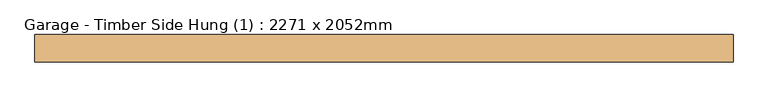
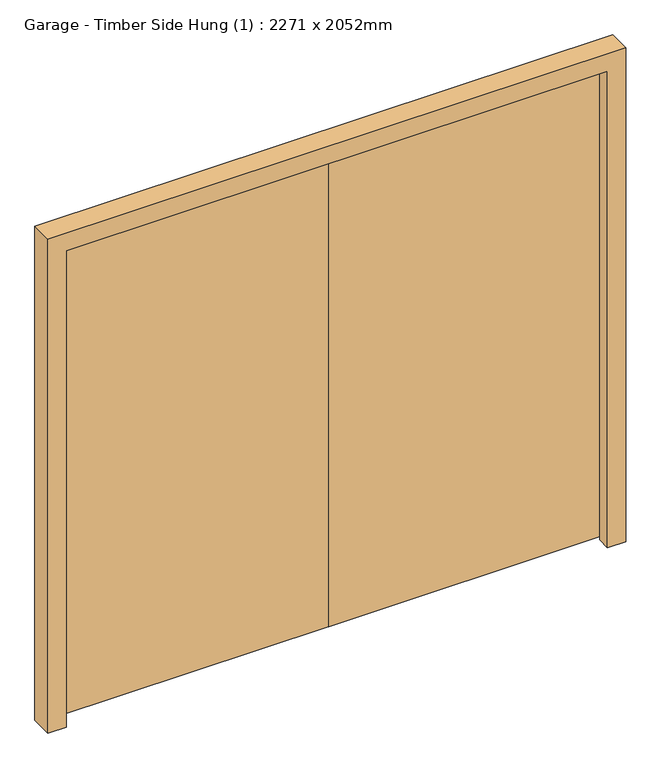
"""IFC4 building model written with IfcOpenShell, lengths in millimetres: door geometry, Garage - Timber Side Hung (1) : 2271 x 2052mm."""

from ifc_helpers import new_model, si_unit, origin, place, context, project, spatial, faceted_brep, source, transform, mapped, element, save


def garage_timber_side_hung_1_2271_x_2052mm_efc604d9(model_context):
    return source(origin(), model_context, "Body", "Brep", [
        faceted_brep([(1085.5, 102.0, 0.0), (1135.5, 102.0, 0.0), (1135.5, 13.0, 0.0), (1063.5, 13.0, 0.0), (1063.5, 67.0, 0.0), (1085.5, 67.0, 0.0), (1085.5, 102.0, 2002.0), (-1085.5, 102.0, 2002.0), (-1085.5, 102.0, 0.0), (-1135.5, 102.0, 0.0), (-1135.5, 102.0, 2052.0), (1135.5, 102.0, 2052.0), (1135.5, 13.0, 2052.0), (-1135.5, 13.0, 2052.0), (-1135.5, 13.0, 0.0), (-1063.5, 13.0, 0.0), (-1063.5, 13.0, 1980.0), (1063.5, 13.0, 1980.0), (1063.5, 67.0, 1980.0), (-1063.5, 67.0, 1980.0), (-1063.5, 67.0, 0.0), (-1085.5, 67.0, 0.0), (-1085.5, 67.0, 2002.0), (1085.5, 67.0, 2002.0)], [[[0, 1, 2, 3, 4, 5]], [[1, 0, 6, 7, 8, 9, 10, 11]], [[2, 1, 11, 12]], [[3, 2, 12, 13, 14, 15, 16, 17]], [[4, 3, 17, 18]], [[5, 4, 18, 19, 20, 21, 22, 23]], [[0, 5, 23, 6]], [[8, 7, 22, 21]], [[9, 8, 21, 20, 15, 14]], [[10, 9, 14, 13]], [[16, 15, 20, 19]], [[11, 10, 13, 12]], [[17, 16, 19, 18]], [[7, 6, 23, 22]]]),
        faceted_brep([(1.5, 70.0, 10.0), (1082.5, 70.0, 10.0), (1082.5, 70.0, 1999.0), (1.5, 70.0, 1999.0), (1.5, 102.0, 10.0), (1.5, 102.0, 1999.0), (1082.5, 102.0, 1999.0), (1082.5, 102.0, 10.0), (101.5, 102.0, 1799.0), (101.5, 102.0, 260.0), (907.5, 102.0, 260.0), (907.5, 102.0, 1799.0), (101.5, 97.0, 260.0), (101.5, 97.0, 1799.0), (907.5, 97.0, 1799.0), (907.5, 97.0, 260.0)], [[[0, 1, 2, 3]], [[4, 5, 6, 7], [8, 9, 10, 11]], [[1, 0, 4, 7]], [[2, 1, 7, 6]], [[3, 2, 6, 5]], [[0, 3, 5, 4]], [[12, 13, 14, 15]], [[13, 12, 9, 8]], [[14, 13, 8, 11]], [[15, 14, 11, 10]], [[12, 15, 10, 9]]]),
        faceted_brep([(-1082.5, 70.0, 10.0), (-1.5, 70.0, 10.0), (-1.5, 70.0, 1999.0), (-1082.5, 70.0, 1999.0), (-1082.5, 102.0, 10.0), (-1082.5, 102.0, 1999.0), (-1.5, 102.0, 1999.0), (-1.5, 102.0, 10.0), (-101.5, 102.0, 1799.0), (-907.5, 102.0, 1799.0), (-907.5, 102.0, 260.0), (-101.5, 102.0, 260.0), (-907.5, 97.0, 1799.0), (-101.5, 97.0, 1799.0), (-101.5, 97.0, 260.0), (-907.5, 97.0, 260.0)], [[[0, 1, 2, 3]], [[4, 5, 6, 7], [8, 9, 10, 11]], [[1, 0, 4, 7]], [[2, 1, 7, 6]], [[3, 2, 6, 5]], [[0, 3, 5, 4]], [[12, 13, 14, 15]], [[13, 12, 9, 8]], [[14, 13, 8, 11]], [[15, 14, 11, 10]], [[12, 15, 10, 9]]]),
    ])


if __name__ == "__main__":
    model = new_model("IFC4")
    model_context = context("Model", 3, world=origin())
    ifc_project = project(units=[si_unit("LENGTHUNIT", "METRE", prefix="MILLI")], contexts=[model_context])
    site = spatial("IfcSite", under=ifc_project)
    building = spatial("IfcBuilding", under=site)
    placement = place(None, origin())
    garage_timber_side_hung_1_2271_x_2052mm_shape = garage_timber_side_hung_1_2271_x_2052mm_efc604d9(model_context)
    element("IfcDoor", 1, ObjectType="Garage - Timber Side Hung (1) : 2271 x 2052mm", at=placement, inside=building, context=model_context, shape_type="MappedRepresentation", body=[
        mapped(garage_timber_side_hung_1_2271_x_2052mm_shape, transform((0.0, 0.0, 0.0), x_axis=(1.0, 0.0, 0.0), y_axis=(0.0, 1.0, 0.0), z_axis=(0.0, 0.0, 1.0))),
    ])
    save(model, "model.ifc")

# Revit data of these elements
# Type "Garage - Timber Side Hung (1) : 2271 x 2052mm"
#   Type Mark = "13"
#   Type Comments = "External Garage"
#   Operation = "DoubleDoorSingleSwing"
#   Manufacturer = "Revit"
#   Keynote = "L20"
#   Wrap Layers (Ext) from Ext = 0' - 4.03543"
#   Wrap Layers (Int) from Ext = 0' - 6.98819"
#   Thickness = 0' - 1.25984"
#   Stile Top Rail = 0' - 7.87402"
#   Stile Shutting = 0' - 3.93701"
#   Stile Lock Rail = 0' - 7.87402"
#   Stile Hanging = 0' - 6.88976"
#   Stile Bottom Rail = 0' - 9.84252"
#   Rough Width = 7' - 5.40945"
#   Rough Height = 6' - 8.7874"
#   O/A Frame Width = 0' - 2.51969"
#   Handle Z Distance = 3' - 5.33858"
#   Glazing Panel Height = 1' - 5.71654"
#   FrameWidth = 0' - 1.65354"
#   FrameOffset - External = 0' - 0.98425"
#   FrameDepth = 0' - 3.50394"
#   Door Panel Thickness = 0' - 1.25984"
#   Height = 6' - 8.7874"
#   Structural Tolerance = 0' - 0.31496"
#   Tolerance = 0' - 0.11811"
#   Undercut = 0' - 0.3937"
#   Width = 7' - 5.40945"
#   Cavity Closer Width = 0' - 1.9685"
#   Cavity Closer Offset from Ext = 0' - 4.03543"
#   Cavity Closer Depth = 0' - 2.95276"
#   Vis - Cavity Closers = yes
#   Function = 1
#   Material Door = Door - Panel
#   Wall Closure = (empty or 0)
# Element 1 (IfcDoor, "Garage - Timber Side Hung (1) : 2271 x 2052mm")
#   Materials on its faces: "Door - Panel"
# Materials
#   "Door - Panel": class "Wood", colour RGB 210 159 95, transparency 0, Cost = 0
